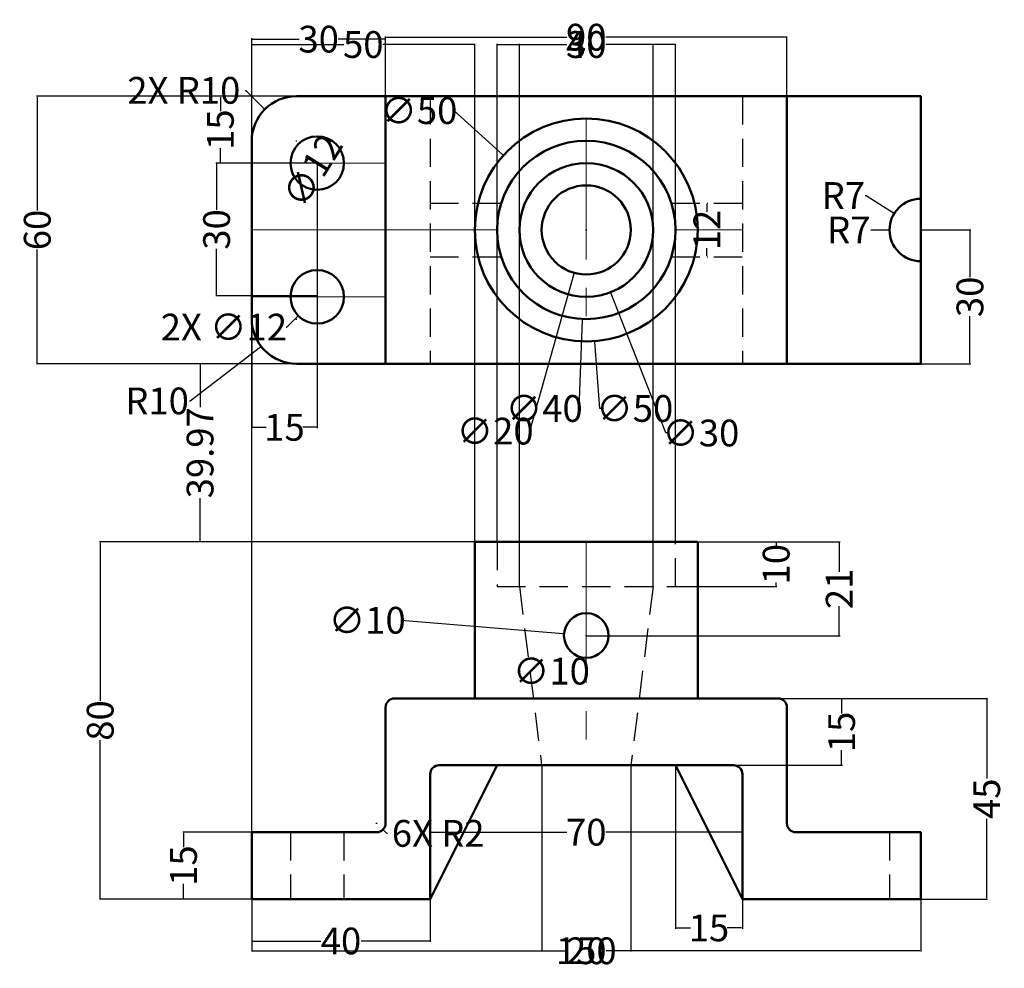
# Model space of a CAD drawing. Units: millimetres. Extents: x 74 to 295, y 59 to 272.
import ezdxf

# ---------------------------------------------------------------- set-up
doc = ezdxf.new("R2010")
doc.units = ezdxf.units.MM
doc.header["$MEASUREMENT"] = 0
doc.linetypes.add('CENTER', pattern=[50.8, 31.75, -6.35, 6.35, -6.35])
doc.linetypes.add('HIDDEN', pattern=[9.525, 6.35, -3.175])
for name, color, linetype, lineweight in [('M-CNTR', 4, 'CENTER', 18), ('M-DIMS', 2, 'Continuous', 25), ('M-HIDN', 3, 'HIDDEN', 25), ('M-OUTL', 7, 'Continuous', 50)]:
    doc.layers.add(name, color=color, linetype=linetype, lineweight=lineweight)
doc.styles.get("Standard").update_dxf_attribs({"font": 'arial.ttf'})
doc.dimstyles.get("Standard").update_dxf_attribs({"dimtxt": 6, "dimasz": 0.18, "dimexe": 0.18, "dimexo": 0.0625, "dimgap": 0.09, "dimtad": 0, "dimtoh": 1, "dimdec": 0, "dimzin": 0, "dimdsep": 46, "dimtxsty": 'Standard', "dimcen": 0.09, "dimadec": 0, "dimazin": 0, "dimtfac": 1, "dimtdec": 0, "dimtofl": 0, "dimtmove": 0, "dimatfit": 3, "dimfxl": 1, "dimtolj": 1, "dimtzin": 0, "dimarcsym": 0})

# ---------------------------------------------------------------- blocks, each defined once
blk = doc.blocks.new('*U1')
at = {"layer": 'M-CNTR', "color": 0, "transparency": 16777216}
blk.add_line((0, 25.12), (0, -25.12), dxfattribs=at)
blk = doc.blocks.new('*D2')
at = {"layer": 'Defpoints', "color": 0, "transparency": 16777216}
for p in [(156.09, 267.91), (126.09, 245.1), (156.09, 245.1)]:
    blk.add_point(p, dxfattribs=at)
at = {"layer": 'M-DIMS', "color": 0, "lineweight": -2, "transparency": 16777216}
for p, q in [((126.09, 245.17), (126.09, 268.09)), ((126.27, 267.91), (136.71, 267.91)), ((155.91, 267.91), (145.46, 267.91)), ((156.09, 245.17), (156.09, 268.09))]:
    blk.add_line(p, q, dxfattribs=at)
at = {"layer": 'M-DIMS', "color": 0, "transparency": 16777216}
for points in [[(126.27, 267.94), (126.27, 267.88), (126.09, 267.91)], [(155.91, 267.94), (155.91, 267.88), (156.09, 267.91)]]:
    blk.add_solid(points, dxfattribs=at)
at = {"layer": 'M-DIMS', "color": 0, "transparency": 16777216, "insert": (141.09, 267.91), "char_height": 6, "attachment_point": 5}
blk.add_mtext('\\A1;30', dxfattribs=at)
blk = doc.blocks.new('*D3')
at = {"layer": 'Defpoints', "color": 0, "transparency": 16777216}
for p in [(246.09, 268.34), (156.09, 255.1), (246.09, 255.1)]:
    blk.add_point(p, dxfattribs=at)
at = {"layer": 'M-DIMS', "color": 0, "lineweight": -2, "transparency": 16777216}
for p, q in [((156.09, 255.17), (156.09, 268.52)), ((156.27, 268.34), (196.71, 268.34)), ((245.91, 268.34), (205.46, 268.34)), ((246.09, 255.17), (246.09, 268.52))]:
    blk.add_line(p, q, dxfattribs=at)
at = {"layer": 'M-DIMS', "color": 0, "transparency": 16777216}
for points in [[(156.27, 268.37), (156.27, 268.31), (156.09, 268.34)], [(245.91, 268.37), (245.91, 268.31), (246.09, 268.34)]]:
    blk.add_solid(points, dxfattribs=at)
at = {"layer": 'M-DIMS', "color": 0, "transparency": 16777216, "insert": (201.09, 268.34), "char_height": 6, "attachment_point": 5}
blk.add_mtext('\\A1;90', dxfattribs=at)
blk = doc.blocks.new('*D4')
at = {"layer": 'Defpoints', "color": 0, "transparency": 16777216}
for p in [(228.13, 231.1), (228.13, 231.1), (228.13, 219.1)]:
    blk.add_point(p, dxfattribs=at)
at = {"layer": 'M-DIMS', "color": 0, "lineweight": -2, "transparency": 16777216}
for p, q in [((228.13, 230.92), (228.13, 229.18)), ((228.19, 231.1), (228.31, 231.1)), ((228.13, 219.28), (228.13, 221.03)), ((228.19, 219.1), (228.31, 219.1))]:
    blk.add_line(p, q, dxfattribs=at)
at = {"layer": 'M-DIMS', "color": 0, "transparency": 16777216}
for points in [[(228.1, 230.92), (228.16, 230.92), (228.13, 231.1)], [(228.1, 219.28), (228.16, 219.28), (228.13, 219.1)]]:
    blk.add_solid(points, dxfattribs=at)
at = {"layer": 'M-DIMS', "color": 0, "transparency": 16777216, "insert": (228.13, 225.1), "char_height": 6, "attachment_point": 5, "rotation": 90}
blk.add_mtext('\\A1;12', dxfattribs=at)
blk = doc.blocks.new('*D5')
at = {"layer": 'Defpoints', "color": 0, "transparency": 16777216}
for p in [(276.09, 225.1), (276.09, 195.1), (287.11, 195.1)]:
    blk.add_point(p, dxfattribs=at)
at = {"layer": 'M-DIMS', "color": 0, "lineweight": -2, "transparency": 16777216}
for p, q in [((276.15, 225.1), (287.29, 225.1)), ((287.11, 224.92), (287.11, 214.48)), ((287.11, 195.28), (287.11, 205.73)), ((276.15, 195.1), (287.29, 195.1))]:
    blk.add_line(p, q, dxfattribs=at)
at = {"layer": 'M-DIMS', "color": 0, "transparency": 16777216}
for points in [[(287.08, 224.92), (287.14, 224.92), (287.11, 225.1)], [(287.08, 195.28), (287.14, 195.28), (287.11, 195.1)]]:
    blk.add_solid(points, dxfattribs=at)
at = {"layer": 'M-DIMS', "color": 0, "transparency": 16777216, "insert": (287.11, 210.1), "char_height": 6, "attachment_point": 5, "rotation": 90}
blk.add_mtext('\\A1;30', dxfattribs=at)
blk = doc.blocks.new('*D6')
at = {"layer": 'Defpoints', "color": 0, "transparency": 16777216}
for p in [(126.09, 240.1), (140.77, 240.1), (126.09, 180.83)]:
    blk.add_point(p, dxfattribs=at)
at = {"layer": 'M-DIMS', "color": 0, "lineweight": -2, "transparency": 16777216}
for p, q in [((126.09, 240.04), (126.09, 180.65)), ((140.77, 240.04), (140.77, 180.65)), ((126.27, 180.83), (129.3, 180.83)), ((140.59, 180.83), (137.55, 180.83))]:
    blk.add_line(p, q, dxfattribs=at)
at = {"layer": 'M-DIMS', "color": 0, "transparency": 16777216}
for points in [[(126.27, 180.86), (126.27, 180.8), (126.09, 180.83)], [(140.59, 180.86), (140.59, 180.8), (140.77, 180.83)]]:
    blk.add_solid(points, dxfattribs=at)
at = {"layer": 'M-DIMS', "color": 0, "transparency": 16777216, "insert": (133.43, 180.83), "char_height": 6, "attachment_point": 5}
blk.add_mtext('\\A1;15', dxfattribs=at)
blk = doc.blocks.new('*D7')
at = {"layer": 'Defpoints', "color": 0, "transparency": 16777216}
for p in [(119.05, 255.1), (141.09, 255.1), (141.09, 240.1)]:
    blk.add_point(p, dxfattribs=at)
at = {"layer": 'M-DIMS', "color": 0, "lineweight": -2, "transparency": 16777216}
for p, q in [((141.02, 255.1), (118.87, 255.1)), ((119.05, 254.92), (119.05, 251.73)), ((119.05, 240.28), (119.05, 243.48)), ((141.02, 240.1), (118.87, 240.1))]:
    blk.add_line(p, q, dxfattribs=at)
at = {"layer": 'M-DIMS', "color": 0, "transparency": 16777216}
for points in [[(119.02, 254.92), (119.08, 254.92), (119.05, 255.1)], [(119.02, 240.28), (119.08, 240.28), (119.05, 240.1)]]:
    blk.add_solid(points, dxfattribs=at)
at = {"layer": 'M-DIMS', "color": 0, "transparency": 16777216, "insert": (119.05, 247.6), "char_height": 6, "attachment_point": 5, "rotation": 90}
blk.add_mtext('\\A1;15', dxfattribs=at)
blk = doc.blocks.new('*D8')
at = {"layer": 'Defpoints', "color": 0, "transparency": 16777216}
for p in [(140.77, 240.1), (118.2, 210.34), (140.77, 210.34)]:
    blk.add_point(p, dxfattribs=at)
at = {"layer": 'M-DIMS', "color": 0, "lineweight": -2, "transparency": 16777216}
for p, q in [((140.7, 240.1), (118.02, 240.1)), ((118.2, 239.92), (118.2, 229.6)), ((118.2, 210.52), (118.2, 220.85)), ((140.7, 210.34), (118.02, 210.34))]:
    blk.add_line(p, q, dxfattribs=at)
at = {"layer": 'M-DIMS', "color": 0, "transparency": 16777216}
for points in [[(118.17, 239.92), (118.23, 239.92), (118.2, 240.1)], [(118.17, 210.52), (118.23, 210.52), (118.2, 210.34)]]:
    blk.add_solid(points, dxfattribs=at)
at = {"layer": 'M-DIMS', "color": 0, "transparency": 16777216, "insert": (118.2, 225.22), "char_height": 6, "attachment_point": 5, "rotation": 90}
blk.add_mtext('\\A1;30', dxfattribs=at)
blk = doc.blocks.new('*D9')
at = {"layer": 'Defpoints', "color": 0, "transparency": 16777216}
for p in [(270.16, 228.83), (276.09, 225.1)]:
    blk.add_point(p, dxfattribs=at)
at = {"layer": 'M-DIMS', "color": 0, "lineweight": -2, "transparency": 16777216}
for p, q in [((263.64, 232.83), (263.82, 232.83)), ((263.82, 232.83), (270.01, 228.93)), ((276.09, 225.01), (276.09, 225.19)), ((276, 225.1), (276.18, 225.1))]:
    blk.add_line(p, q, dxfattribs=at)
at = {"layer": 'M-DIMS', "color": 0, "transparency": 16777216}
blk.add_solid([(270.03, 228.95), (270, 228.9), (270.16, 228.83)], dxfattribs=at)
at = {"layer": 'M-DIMS', "color": 0, "transparency": 16777216, "insert": (258.72, 232.83), "char_height": 6, "attachment_point": 5}
blk.add_mtext('\\A1;R7', dxfattribs=at)
blk = doc.blocks.new('*D10')
at = {"layer": 'Defpoints', "color": 0, "transparency": 16777216}
for p in [(143.95, 245.19), (137.58, 235.02)]:
    blk.add_point(p, dxfattribs=at)
at = {"layer": 'M-DIMS', "color": 0, "lineweight": -2, "transparency": 16777216}
blk.add_line((143.76, 244.88), (143.85, 245.04), dxfattribs=at)
at = {"layer": 'M-DIMS', "color": 0, "transparency": 16777216}
blk.add_solid([(143.83, 245.05), (143.88, 245.02), (143.95, 245.19)], dxfattribs=at)
at = {"layer": 'M-DIMS', "color": 0, "transparency": 16777216, "insert": (139.72, 238.42), "char_height": 6, "attachment_point": 5, "rotation": 57.9702}
blk.add_mtext('\\A1;∅12', dxfattribs=at)
blk = doc.blocks.new('*D11')
at = {"layer": 'Defpoints', "color": 0, "transparency": 16777216}
for p in [(136.09, 255.1), (77.99, 195.1), (136.09, 195.1)]:
    blk.add_point(p, dxfattribs=at)
at = {"layer": 'M-DIMS', "color": 0, "lineweight": -2, "transparency": 16777216}
for p, q in [((136.02, 255.1), (77.81, 255.1)), ((77.99, 254.92), (77.99, 229.5)), ((77.99, 195.28), (77.99, 220.71)), ((136.02, 195.1), (77.81, 195.1))]:
    blk.add_line(p, q, dxfattribs=at)
at = {"layer": 'M-DIMS', "color": 0, "transparency": 16777216}
for points in [[(77.96, 254.92), (78.02, 254.92), (77.99, 255.1)], [(77.96, 195.28), (78.02, 195.28), (77.99, 195.1)]]:
    blk.add_solid(points, dxfattribs=at)
at = {"layer": 'M-DIMS', "color": 0, "transparency": 16777216, "insert": (77.99, 225.1), "char_height": 6, "attachment_point": 5, "rotation": 90}
blk.add_mtext('\\A1;60', dxfattribs=at)
blk = doc.blocks.new('*D12')
at = {"layer": 'Defpoints', "color": 0, "transparency": 16777216}
for p in [(203.78, 234.73), (198.4, 215.47)]:
    blk.add_point(p, dxfattribs=at)
at = {"layer": 'M-DIMS', "color": 0, "lineweight": -2, "transparency": 16777216}
for p, q in [((201.09, 225.01), (201.09, 225.19)), ((201, 225.1), (201.18, 225.1)), ((188.47, 179.98), (198.35, 215.3)), ((188.29, 179.98), (188.47, 179.98))]:
    blk.add_line(p, q, dxfattribs=at)
at = {"layer": 'M-DIMS', "color": 0, "transparency": 16777216}
blk.add_solid([(198.32, 215.31), (198.38, 215.29), (198.4, 215.47)], dxfattribs=at)
at = {"layer": 'M-DIMS', "color": 0, "transparency": 16777216, "insert": (180.65, 179.98), "char_height": 6, "attachment_point": 5}
blk.add_mtext('\\A1;∅20', dxfattribs=at)
blk = doc.blocks.new('*D13')
at = {"layer": 'Defpoints', "color": 0, "transparency": 16777216}
for p in [(195.61, 239.07), (206.57, 211.14)]:
    blk.add_point(p, dxfattribs=at)
at = {"layer": 'M-DIMS', "color": 0, "lineweight": -2, "transparency": 16777216}
for p, q in [((201.09, 225.01), (201.09, 225.19)), ((201, 225.1), (201.18, 225.1)), ((218.95, 179.56), (206.63, 210.97)), ((219.13, 179.56), (218.95, 179.56))]:
    blk.add_line(p, q, dxfattribs=at)
at = {"layer": 'M-DIMS', "color": 0, "transparency": 16777216}
blk.add_solid([(206.66, 210.98), (206.6, 210.96), (206.57, 211.14)], dxfattribs=at)
at = {"layer": 'M-DIMS', "color": 0, "transparency": 16777216, "insert": (226.77, 179.56), "char_height": 6, "attachment_point": 5}
blk.add_mtext('\\A1;∅30', dxfattribs=at)
blk = doc.blocks.new('*D14')
at = {"layer": 'Defpoints', "color": 0, "transparency": 16777216}
for p in [(201.89, 245.09), (200.29, 205.12)]:
    blk.add_point(p, dxfattribs=at)
at = {"layer": 'M-DIMS', "color": 0, "lineweight": -2, "transparency": 16777216}
for p, q in [((201.09, 225.01), (201.09, 225.19)), ((201, 225.1), (201.18, 225.1)), ((199.48, 185.06), (200.28, 204.94)), ((199.3, 185.06), (199.48, 185.06))]:
    blk.add_line(p, q, dxfattribs=at)
at = {"layer": 'M-DIMS', "color": 0, "transparency": 16777216}
blk.add_solid([(200.25, 204.94), (200.31, 204.94), (200.29, 205.12)], dxfattribs=at)
at = {"layer": 'M-DIMS', "color": 0, "transparency": 16777216, "insert": (191.66, 185.06), "char_height": 6, "attachment_point": 5}
blk.add_mtext('\\A1;∅40', dxfattribs=at)
blk = doc.blocks.new('*D15')
at = {"layer": 'Defpoints', "color": 0, "transparency": 16777216}
for p in [(199.19, 250.03), (202.99, 200.17)]:
    blk.add_point(p, dxfattribs=at)
at = {"layer": 'M-DIMS', "color": 0, "lineweight": -2, "transparency": 16777216}
for p, q in [((201.09, 225.01), (201.09, 225.19)), ((201, 225.1), (201.18, 225.1)), ((204.14, 185.06), (203, 200)), ((204.32, 185.06), (204.14, 185.06))]:
    blk.add_line(p, q, dxfattribs=at)
at = {"layer": 'M-DIMS', "color": 0, "transparency": 16777216}
blk.add_solid([(203.03, 200), (202.97, 199.99), (202.99, 200.17)], dxfattribs=at)
at = {"layer": 'M-DIMS', "color": 0, "transparency": 16777216, "insert": (211.96, 185.06), "char_height": 6, "attachment_point": 5}
blk.add_mtext('\\A1;∅50', dxfattribs=at)
blk = doc.blocks.new('*D16')
at = {"layer": 'Defpoints', "color": 0, "transparency": 16777216}
for p in [(136.09, 205.1), (128.17, 199)]:
    blk.add_point(p, dxfattribs=at)
at = {"layer": 'M-DIMS', "color": 0, "lineweight": -2, "transparency": 16777216}
for p, q in [((136, 205.1), (136.18, 205.1)), ((136.09, 205.01), (136.09, 205.19)), ((112.28, 186.75), (128.02, 198.89)), ((112.1, 186.75), (112.28, 186.75))]:
    blk.add_line(p, q, dxfattribs=at)
at = {"layer": 'M-DIMS', "color": 0, "transparency": 16777216}
blk.add_solid([(128.01, 198.91), (128.04, 198.86), (128.17, 199)], dxfattribs=at)
at = {"layer": 'M-DIMS', "color": 0, "transparency": 16777216, "insert": (104.85, 186.75), "char_height": 6, "attachment_point": 5}
blk.add_mtext('\\A1;R10', dxfattribs=at)
blk = doc.blocks.new('*D17')
at = {"layer": 'Defpoints', "color": 0, "transparency": 16777216}
for p in [(196.1, 134.54), (206.07, 133.72)]:
    blk.add_point(p, dxfattribs=at)
at = {"layer": 'M-DIMS', "color": 0, "lineweight": -2, "transparency": 16777216}
for p, q in [((159.61, 137.55), (195.92, 134.56)), ((201, 134.13), (201.18, 134.13)), ((201.09, 134.04), (201.09, 134.22))]:
    blk.add_line(p, q, dxfattribs=at)
at = {"layer": 'M-DIMS', "color": 0, "transparency": 16777216}
blk.add_solid([(195.93, 134.59), (195.92, 134.53), (196.1, 134.54)], dxfattribs=at)
at = {"layer": 'M-DIMS', "color": 0, "transparency": 16777216, "insert": (151.97, 137.55), "char_height": 6, "attachment_point": 5}
blk.add_mtext('\\A1;∅10', dxfattribs=at)
blk = doc.blocks.new('*D18')
at = {"layer": 'Defpoints', "color": 0, "transparency": 16777216}
for p in [(221.09, 155.13), (243.66, 155.13), (221.09, 145.13)]:
    blk.add_point(p, dxfattribs=at)
at = {"layer": 'M-DIMS', "color": 0, "lineweight": -2, "transparency": 16777216}
for p, q in [((221.15, 155.13), (243.84, 155.13)), ((243.66, 154.95), (243.66, 154.23)), ((243.66, 145.31), (243.66, 146.04)), ((221.15, 145.13), (243.84, 145.13))]:
    blk.add_line(p, q, dxfattribs=at)
at = {"layer": 'M-DIMS', "color": 0, "transparency": 16777216}
for points in [[(243.63, 154.95), (243.69, 154.95), (243.66, 155.13)], [(243.63, 145.31), (243.69, 145.31), (243.66, 145.13)]]:
    blk.add_solid(points, dxfattribs=at)
at = {"layer": 'M-DIMS', "color": 0, "transparency": 16777216, "insert": (243.66, 150.13), "char_height": 6, "attachment_point": 5, "rotation": 90}
blk.add_mtext('\\A1;10', dxfattribs=at)
blk = doc.blocks.new('*D19')
at = {"layer": 'Defpoints', "color": 0, "transparency": 16777216}
for p in [(201.09, 155.13), (257.8, 155.13), (201.09, 134.04)]:
    blk.add_point(p, dxfattribs=at)
at = {"layer": 'M-DIMS', "color": 0, "lineweight": -2, "transparency": 16777216}
for p, q in [((201.15, 155.13), (257.98, 155.13)), ((257.8, 154.95), (257.8, 148.45)), ((257.8, 134.22), (257.8, 140.73)), ((201.15, 134.04), (257.98, 134.04))]:
    blk.add_line(p, q, dxfattribs=at)
at = {"layer": 'M-DIMS', "color": 0, "transparency": 16777216}
for points in [[(257.77, 154.95), (257.83, 154.95), (257.8, 155.13)], [(257.77, 134.22), (257.83, 134.22), (257.8, 134.04)]]:
    blk.add_solid(points, dxfattribs=at)
at = {"layer": 'M-DIMS', "color": 0, "transparency": 16777216, "insert": (257.8, 144.59), "char_height": 6, "attachment_point": 5, "rotation": 90}
blk.add_mtext('\\A1;21', dxfattribs=at)
blk = doc.blocks.new('*D20')
at = {"layer": 'Defpoints', "color": 0, "transparency": 16777216}
for p in [(234.09, 120.01), (258.33, 120.01), (234.09, 105.01)]:
    blk.add_point(p, dxfattribs=at)
at = {"layer": 'M-DIMS', "color": 0, "lineweight": -2, "transparency": 16777216}
for p, q in [((234.15, 120.01), (258.51, 120.01)), ((258.33, 119.83), (258.33, 116.64)), ((258.33, 105.19), (258.33, 108.39)), ((234.15, 105.01), (258.51, 105.01))]:
    blk.add_line(p, q, dxfattribs=at)
at = {"layer": 'M-DIMS', "color": 0, "transparency": 16777216}
for points in [[(258.3, 119.83), (258.36, 119.83), (258.33, 120.01)], [(258.3, 105.19), (258.36, 105.19), (258.33, 105.01)]]:
    blk.add_solid(points, dxfattribs=at)
at = {"layer": 'M-DIMS', "color": 0, "transparency": 16777216, "insert": (258.33, 112.51), "char_height": 6, "attachment_point": 5, "rotation": 90}
blk.add_mtext('\\A1;15', dxfattribs=at)
blk = doc.blocks.new('*D21')
at = {"layer": 'Defpoints', "color": 0, "transparency": 16777216}
for p in [(126.09, 75.01), (166.09, 75.01), (166.09, 65.6)]:
    blk.add_point(p, dxfattribs=at)
at = {"layer": 'M-DIMS', "color": 0, "lineweight": -2, "transparency": 16777216}
for p, q in [((126.09, 74.95), (126.09, 65.42)), ((166.09, 74.95), (166.09, 65.42)), ((126.27, 65.6), (141.59, 65.6)), ((165.91, 65.6), (150.59, 65.6))]:
    blk.add_line(p, q, dxfattribs=at)
at = {"layer": 'M-DIMS', "color": 0, "transparency": 16777216}
for points in [[(126.27, 65.63), (126.27, 65.57), (126.09, 65.6)], [(165.91, 65.63), (165.91, 65.57), (166.09, 65.6)]]:
    blk.add_solid(points, dxfattribs=at)
at = {"layer": 'M-DIMS', "color": 0, "transparency": 16777216, "insert": (146.09, 65.6), "char_height": 6, "attachment_point": 5}
blk.add_mtext('\\A1;40', dxfattribs=at)
blk = doc.blocks.new('*D22')
at = {"layer": 'Defpoints', "color": 0, "transparency": 16777216}
for p in [(221.09, 105.01), (236.09, 89.01), (236.09, 68.54)]:
    blk.add_point(p, dxfattribs=at)
at = {"layer": 'M-DIMS', "color": 0, "lineweight": -2, "transparency": 16777216}
for p, q in [((221.09, 104.95), (221.09, 68.36)), ((236.09, 88.95), (236.09, 68.36)), ((221.27, 68.54), (224.46, 68.54)), ((235.91, 68.54), (232.71, 68.54))]:
    blk.add_line(p, q, dxfattribs=at)
at = {"layer": 'M-DIMS', "color": 0, "transparency": 16777216}
for points in [[(221.27, 68.57), (221.27, 68.51), (221.09, 68.54)], [(235.91, 68.57), (235.91, 68.51), (236.09, 68.54)]]:
    blk.add_solid(points, dxfattribs=at)
at = {"layer": 'M-DIMS', "color": 0, "transparency": 16777216, "insert": (228.59, 68.54), "char_height": 6, "attachment_point": 5}
blk.add_mtext('\\A1;15', dxfattribs=at)
blk = doc.blocks.new('*D23')
at = {"layer": 'Defpoints', "color": 0, "transparency": 16777216}
for p in [(244.09, 120.01), (244.09, 75.01), (290.88, 75.01)]:
    blk.add_point(p, dxfattribs=at)
at = {"layer": 'M-DIMS', "color": 0, "lineweight": -2, "transparency": 16777216}
for p, q in [((244.15, 120.01), (291.06, 120.01)), ((290.88, 119.83), (290.88, 102.04)), ((290.88, 75.19), (290.88, 92.98)), ((244.15, 75.01), (291.06, 75.01))]:
    blk.add_line(p, q, dxfattribs=at)
at = {"layer": 'M-DIMS', "color": 0, "transparency": 16777216}
for points in [[(290.85, 119.83), (290.91, 119.83), (290.88, 120.01)], [(290.85, 75.19), (290.91, 75.19), (290.88, 75.01)]]:
    blk.add_solid(points, dxfattribs=at)
at = {"layer": 'M-DIMS', "color": 0, "transparency": 16777216, "insert": (290.88, 97.51), "char_height": 6, "attachment_point": 5, "rotation": 90}
blk.add_mtext('\\A1;45', dxfattribs=at)
blk = doc.blocks.new('*D24')
at = {"layer": 'Defpoints', "color": 0, "transparency": 16777216}
for p in [(126.09, 90.01), (110.78, 75.01), (126.09, 75.01)]:
    blk.add_point(p, dxfattribs=at)
at = {"layer": 'M-DIMS', "color": 0, "lineweight": -2, "transparency": 16777216}
for p, q in [((126.02, 90.01), (110.6, 90.01)), ((110.78, 89.83), (110.78, 86.64)), ((110.78, 75.19), (110.78, 78.39)), ((126.02, 75.01), (110.6, 75.01))]:
    blk.add_line(p, q, dxfattribs=at)
at = {"layer": 'M-DIMS', "color": 0, "transparency": 16777216}
for points in [[(110.75, 89.83), (110.81, 89.83), (110.78, 90.01)], [(110.75, 75.19), (110.81, 75.19), (110.78, 75.01)]]:
    blk.add_solid(points, dxfattribs=at)
at = {"layer": 'M-DIMS', "color": 0, "transparency": 16777216, "insert": (110.78, 82.51), "char_height": 6, "attachment_point": 5, "rotation": 90}
blk.add_mtext('\\A1;15', dxfattribs=at)
blk = doc.blocks.new('*D25')
at = {"layer": 'Defpoints', "color": 0, "transparency": 16777216}
for p in [(236.09, 90.01), (166.09, 75.01), (236.09, 75.01)]:
    blk.add_point(p, dxfattribs=at)
at = {"layer": 'M-DIMS', "color": 0, "lineweight": -2, "transparency": 16777216}
for p, q in [((166.09, 75.08), (166.09, 90.19)), ((166.27, 90.01), (196.73, 90.01)), ((235.91, 90.01), (205.44, 90.01)), ((236.09, 75.08), (236.09, 90.19))]:
    blk.add_line(p, q, dxfattribs=at)
at = {"layer": 'M-DIMS', "color": 0, "transparency": 16777216}
for points in [[(166.27, 90.04), (166.27, 89.98), (166.09, 90.01)], [(235.91, 90.04), (235.91, 89.98), (236.09, 90.01)]]:
    blk.add_solid(points, dxfattribs=at)
at = {"layer": 'M-DIMS', "color": 0, "transparency": 16777216, "insert": (201.09, 90.01), "char_height": 6, "attachment_point": 5}
blk.add_mtext('\\A1;70', dxfattribs=at)
blk = doc.blocks.new('*D26')
at = {"layer": 'Defpoints', "color": 0, "transparency": 16777216}
for p in [(176.09, 155.13), (92.1, 75.01), (166.09, 75.01)]:
    blk.add_point(p, dxfattribs=at)
at = {"layer": 'M-DIMS', "color": 0, "lineweight": -2, "transparency": 16777216}
for p, q in [((176.02, 155.13), (91.92, 155.13)), ((92.1, 154.95), (92.1, 119.45)), ((92.1, 75.19), (92.1, 110.69)), ((166.02, 75.01), (91.92, 75.01))]:
    blk.add_line(p, q, dxfattribs=at)
at = {"layer": 'M-DIMS', "color": 0, "transparency": 16777216}
for points in [[(92.07, 154.95), (92.13, 154.95), (92.1, 155.13)], [(92.07, 75.19), (92.13, 75.19), (92.1, 75.01)]]:
    blk.add_solid(points, dxfattribs=at)
at = {"layer": 'M-DIMS', "color": 0, "transparency": 16777216, "insert": (92.1, 115.07), "char_height": 6, "attachment_point": 5, "rotation": 90}
blk.add_mtext('\\A1;80', dxfattribs=at)
blk = doc.blocks.new('MOUNT-HOLE-D12')
blk.add_circle((0, 0), 6)
blk = doc.blocks.new('*D28')
at = {"layer": 'Defpoints', "color": 0, "transparency": 16777216}
for p in [(126.09, 75.01), (276.09, 75.01), (276.09, 63.41)]:
    blk.add_point(p, dxfattribs=at)
at = {"layer": 'M-DIMS', "color": 0, "lineweight": -2, "transparency": 16777216}
for p, q in [((126.09, 74.95), (126.09, 63.23)), ((276.09, 74.95), (276.09, 63.23)), ((126.27, 63.41), (194.66, 63.41)), ((275.91, 63.41), (207.51, 63.41))]:
    blk.add_line(p, q, dxfattribs=at)
at = {"layer": 'M-DIMS', "color": 0, "transparency": 16777216}
for points in [[(126.27, 63.44), (126.27, 63.38), (126.09, 63.41)], [(275.91, 63.44), (275.91, 63.38), (276.09, 63.41)]]:
    blk.add_solid(points, dxfattribs=at)
at = {"layer": 'M-DIMS', "color": 0, "transparency": 16777216, "insert": (201.09, 63.41), "char_height": 6, "attachment_point": 5}
blk.add_mtext('\\A1;150', dxfattribs=at)
blk = doc.blocks.new('*D29')
at = {"layer": 'Defpoints', "color": 0, "transparency": 16777216}
for p in [(126.09, 266.7), (176.09, 155.13), (126.09, 90.01)]:
    blk.add_point(p, dxfattribs=at)
at = {"layer": 'M-DIMS', "color": 0, "lineweight": -2, "transparency": 16777216}
for p, q in [((126.09, 90.08), (126.09, 266.88)), ((126.27, 266.7), (146.71, 266.7)), ((175.91, 266.7), (155.46, 266.7)), ((176.09, 155.2), (176.09, 266.88))]:
    blk.add_line(p, q, dxfattribs=at)
at = {"layer": 'M-DIMS', "color": 0, "transparency": 16777216}
for points in [[(126.27, 266.73), (126.27, 266.67), (126.09, 266.7)], [(175.91, 266.73), (175.91, 266.67), (176.09, 266.7)]]:
    blk.add_solid(points, dxfattribs=at)
at = {"layer": 'M-DIMS', "color": 0, "transparency": 16777216, "insert": (151.09, 266.7), "char_height": 6, "attachment_point": 5}
blk.add_mtext('\\A1;50', dxfattribs=at)
blk = doc.blocks.new('*D30')
at = {"layer": 'Defpoints', "color": 0, "transparency": 16777216}
for p in [(221.09, 266.7), (181.09, 155.13), (221.09, 155.13)]:
    blk.add_point(p, dxfattribs=at)
at = {"layer": 'M-DIMS', "color": 0, "lineweight": -2, "transparency": 16777216}
for p, q in [((181.09, 155.2), (181.09, 266.88)), ((181.27, 266.7), (196.59, 266.7)), ((220.91, 266.7), (205.59, 266.7)), ((221.09, 155.2), (221.09, 266.88))]:
    blk.add_line(p, q, dxfattribs=at)
at = {"layer": 'M-DIMS', "color": 0, "transparency": 16777216}
for points in [[(181.27, 266.73), (181.27, 266.67), (181.09, 266.7)], [(220.91, 266.73), (220.91, 266.67), (221.09, 266.7)]]:
    blk.add_solid(points, dxfattribs=at)
at = {"layer": 'M-DIMS', "color": 0, "transparency": 16777216, "insert": (201.09, 266.7), "char_height": 6, "attachment_point": 5}
blk.add_mtext('\\A1;40', dxfattribs=at)
blk = doc.blocks.new('*D31')
at = {"layer": 'Defpoints', "color": 0, "transparency": 16777216}
for p in [(216.09, 266.7), (186.09, 145.13), (216.09, 145.13)]:
    blk.add_point(p, dxfattribs=at)
at = {"layer": 'M-DIMS', "color": 0, "lineweight": -2, "transparency": 16777216}
for p, q in [((186.09, 145.2), (186.09, 266.88)), ((186.27, 266.7), (196.71, 266.7)), ((215.91, 266.7), (205.46, 266.7)), ((216.09, 145.2), (216.09, 266.88))]:
    blk.add_line(p, q, dxfattribs=at)
at = {"layer": 'M-DIMS', "color": 0, "transparency": 16777216}
for points in [[(186.27, 266.73), (186.27, 266.67), (186.09, 266.7)], [(215.91, 266.73), (215.91, 266.67), (216.09, 266.7)]]:
    blk.add_solid(points, dxfattribs=at)
at = {"layer": 'M-DIMS', "color": 0, "transparency": 16777216, "insert": (201.09, 266.7), "char_height": 6, "attachment_point": 5}
blk.add_mtext('\\A1;30', dxfattribs=at)
blk = doc.blocks.new('*D32')
at = {"layer": 'Defpoints', "color": 0, "transparency": 16777216}
for p in [(191.09, 105.01), (211.09, 105.01), (211.09, 63.41)]:
    blk.add_point(p, dxfattribs=at)
at = {"layer": 'M-DIMS', "color": 0, "lineweight": -2, "transparency": 16777216}
for p, q in [((191.09, 104.95), (191.09, 63.23)), ((211.09, 104.95), (211.09, 63.23)), ((191.27, 63.41), (196.66, 63.41)), ((210.91, 63.41), (205.52, 63.41))]:
    blk.add_line(p, q, dxfattribs=at)
at = {"layer": 'M-DIMS', "color": 0, "transparency": 16777216}
for points in [[(191.27, 63.44), (191.27, 63.38), (191.09, 63.41)], [(210.91, 63.44), (210.91, 63.38), (211.09, 63.41)]]:
    blk.add_solid(points, dxfattribs=at)
at = {"layer": 'M-DIMS', "color": 0, "transparency": 16777216, "insert": (201.09, 63.41), "char_height": 6, "attachment_point": 5}
blk.add_mtext('\\A1;20', dxfattribs=at)
blk = doc.blocks.new('*D33')
at = {"layer": 'Defpoints', "color": 0, "transparency": 16777216}
for p in [(156.09, 195.1), (114.49, 155.13), (176.09, 155.13)]:
    blk.add_point(p, dxfattribs=at)
at = {"layer": 'M-DIMS', "color": 0, "lineweight": -2, "transparency": 16777216}
for p, q in [((156.02, 195.1), (114.31, 195.1)), ((114.49, 194.92), (114.49, 185.33)), ((114.49, 155.31), (114.49, 164.91)), ((176.02, 155.13), (114.31, 155.13))]:
    blk.add_line(p, q, dxfattribs=at)
at = {"layer": 'M-DIMS', "color": 0, "transparency": 16777216}
for points in [[(114.46, 194.92), (114.52, 194.92), (114.49, 195.1)], [(114.46, 155.31), (114.52, 155.31), (114.49, 155.13)]]:
    blk.add_solid(points, dxfattribs=at)
at = {"layer": 'M-DIMS', "color": 0, "transparency": 16777216, "insert": (114.49, 175.12), "char_height": 6, "attachment_point": 5, "rotation": 90}
blk.add_mtext('\\A1;39.97', dxfattribs=at)
blk = doc.blocks.new('*D34')
at = {"layer": 'Defpoints', "color": 0, "transparency": 16777216}
for p in [(182.52, 241.84), (219.66, 208.36)]:
    blk.add_point(p, dxfattribs=at)
at = {"layer": 'M-DIMS', "color": 0, "lineweight": -2, "transparency": 16777216}
for p, q in [((171.2, 251.88), (171.38, 251.88)), ((171.38, 251.88), (182.38, 241.96)), ((201.09, 225.01), (201.09, 225.19)), ((201, 225.1), (201.18, 225.1))]:
    blk.add_line(p, q, dxfattribs=at)
at = {"layer": 'M-DIMS', "color": 0, "transparency": 16777216}
blk.add_solid([(182.4, 241.98), (182.36, 241.94), (182.52, 241.84)], dxfattribs=at)
at = {"layer": 'M-DIMS', "color": 0, "transparency": 16777216, "insert": (163.56, 251.88), "char_height": 6, "attachment_point": 5}
blk.add_mtext('\\A1;∅50', dxfattribs=at)
blk = doc.blocks.new('*D35')
at = {"layer": 'Defpoints', "color": 0, "transparency": 16777216}
for p in [(129.02, 252.17), (136.09, 245.1)]:
    blk.add_point(p, dxfattribs=at)
at = {"layer": 'M-DIMS', "color": 0, "lineweight": -2, "transparency": 16777216}
for p, q in [((124.59, 256.42), (124.77, 256.42)), ((124.77, 256.42), (128.89, 252.3)), ((136, 245.1), (136.18, 245.1)), ((136.09, 245.01), (136.09, 245.19))]:
    blk.add_line(p, q, dxfattribs=at)
at = {"layer": 'M-DIMS', "color": 0, "transparency": 16777216}
blk.add_solid([(128.91, 252.32), (128.87, 252.28), (129.02, 252.17)], dxfattribs=at)
at = {"layer": 'M-DIMS', "color": 0, "transparency": 16777216, "insert": (110.85, 256.42), "char_height": 6, "attachment_point": 5}
blk.add_mtext('\\A1;2X R10', dxfattribs=at)
blk = doc.blocks.new('*D36')
at = {"layer": 'Defpoints', "color": 0, "transparency": 16777216}
for p in [(269.09, 225.1), (276.09, 225.1)]:
    blk.add_point(p, dxfattribs=at)
at = {"layer": 'M-DIMS', "color": 0, "lineweight": -2, "transparency": 16777216}
for p, q in [((276.09, 225.01), (276.09, 225.19)), ((264.89, 225.1), (268.91, 225.1)), ((276, 225.1), (276.18, 225.1))]:
    blk.add_line(p, q, dxfattribs=at)
at = {"layer": 'M-DIMS', "color": 0, "transparency": 16777216}
blk.add_solid([(268.91, 225.13), (268.91, 225.07), (269.09, 225.1)], dxfattribs=at)
at = {"layer": 'M-DIMS', "color": 0, "transparency": 16777216, "insert": (259.96, 225.1), "char_height": 6, "attachment_point": 5}
blk.add_mtext('\\A1;R7', dxfattribs=at)
blk = doc.blocks.new('*D37')
at = {"layer": 'Defpoints', "color": 0, "transparency": 16777216}
for p in [(145.01, 214.35), (136.52, 205.86)]:
    blk.add_point(p, dxfattribs=at)
at = {"layer": 'M-DIMS', "color": 0, "lineweight": -2, "transparency": 16777216}
for p, q in [((140.68, 210.1), (140.86, 210.1)), ((140.77, 210.01), (140.77, 210.19)), ((133.98, 203.31), (136.4, 205.73)), ((133.8, 203.31), (133.98, 203.31))]:
    blk.add_line(p, q, dxfattribs=at)
at = {"layer": 'M-DIMS', "color": 0, "transparency": 16777216}
blk.add_solid([(136.38, 205.75), (136.42, 205.71), (136.52, 205.86)], dxfattribs=at)
at = {"layer": 'M-DIMS', "color": 0, "transparency": 16777216, "insert": (119.84, 203.31), "char_height": 6, "attachment_point": 5}
blk.add_mtext('\\A1;2X ∅12', dxfattribs=at)
blk = doc.blocks.new('*D38')
at = {"layer": 'Defpoints', "color": 0, "transparency": 16777216}
for p in [(201.09, 139.13), (201.09, 129.13)]:
    blk.add_point(p, dxfattribs=at)
at = {"layer": 'M-DIMS', "color": 0, "lineweight": -2, "transparency": 16777216}
for p, q in [((201, 134.13), (201.18, 134.13)), ((201.09, 134.04), (201.09, 134.22)), ((201.09, 126.13), (201.09, 128.95)), ((200.91, 126.13), (201.09, 126.13))]:
    blk.add_line(p, q, dxfattribs=at)
at = {"layer": 'M-DIMS', "color": 0, "transparency": 16777216}
blk.add_solid([(201.06, 128.95), (201.12, 128.95), (201.09, 129.13)], dxfattribs=at)
at = {"layer": 'M-DIMS', "color": 0, "transparency": 16777216, "insert": (193.27, 126.13), "char_height": 6, "attachment_point": 5}
blk.add_mtext('\\A1;∅10', dxfattribs=at)
blk = doc.blocks.new('*D39')
at = {"layer": 'Defpoints', "color": 0, "transparency": 16777216}
for p in [(154.09, 92.01), (155.5, 90.6)]:
    blk.add_point(p, dxfattribs=at)
at = {"layer": 'M-DIMS', "color": 0, "lineweight": -2, "transparency": 16777216}
for p, q in [((154, 92.01), (154.18, 92.01)), ((154.09, 91.92), (154.09, 92.1)), ((156.35, 89.75), (155.63, 90.47)), ((156.53, 89.75), (156.35, 89.75))]:
    blk.add_line(p, q, dxfattribs=at)
at = {"layer": 'M-DIMS', "color": 0, "transparency": 16777216}
blk.add_solid([(155.65, 90.49), (155.61, 90.45), (155.5, 90.6)], dxfattribs=at)
at = {"layer": 'M-DIMS', "color": 0, "transparency": 16777216, "insert": (167.89, 89.75), "char_height": 6, "attachment_point": 5}
blk.add_mtext('\\A1;6X R2', dxfattribs=at)

msp = doc.modelspace()

# ---------------------------------------------------------------- linework, layer by layer
at = {"layer": 'M-CNTR'}
for p, q in [((126.087, 240.103), (156.087, 240.103)), ((276.087, 240.103), (276.207, 240.103)), ((221.087, 225.103), (236.087, 225.103)), ((221.087, 225.103), (221.087, 225.103)), ((126.087, 210.103), (156.087, 210.103)), ((276.087, 210.103), (276.207, 210.103)), ((201.087, 155.253), (201.087, 105.013))]:
    msp.add_line(p, q, dxfattribs=at)
msp.add_lwpolyline([(126.087, 225.103), (156.087, 225.103), (181.087, 225.103)], dxfattribs=at)
at = {"layer": 'M-HIDN'}
for p, q in [((166.087, 255.103), (166.087, 195.103)), ((236.087, 255.103), (236.087, 195.103)), ((166.087, 231.103), (182.009, 231.103)), ((220.166, 231.103), (236.087, 231.103)), ((166.087, 219.103), (182.009, 219.103)), ((220.166, 219.103), (236.087, 219.103)), ((186.087, 145.133), (191.087, 105.013)), ((216.087, 145.133), (211.087, 105.013)), ((134.767, 90.013), (134.767, 75.013)), ((146.767, 90.013), (146.767, 75.013)), ((269.087, 90.013), (269.087, 75.013))]:
    msp.add_line(p, q, dxfattribs=at)
msp.add_lwpolyline([(181.087, 155.133), (181.087, 145.133), (221.087, 145.133), (221.087, 155.133)], dxfattribs=at)
at = {"layer": 'M-OUTL'}
for p, q in [((156.087, 255.103), (156.087, 195.103)), ((246.087, 255.103), (246.087, 195.103)), ((166.087, 75.013), (181.087, 105.013)), ((236.087, 75.013), (221.087, 105.013))]:
    msp.add_line(p, q, dxfattribs=at)
for points in [[(136.087, 255.103, 0.4142136), (126.087, 245.103), (126.087, 205.103, 0.4142136), (136.087, 195.103), (276.087, 195.103), (276.087, 255.103)], [(276.087, 75.013), (236.087, 75.013), (236.087, 103.013, 0.4142136), (234.087, 105.013), (168.087, 105.013, 0.4142136), (166.087, 103.013), (166.087, 75.013), (126.087, 75.013), (126.087, 90.013), (154.087, 90.013, 0.4142136), (156.087, 92.013), (156.087, 118.013, -0.4142136), (158.087, 120.013), (201.087, 120.013), (244.087, 120.013, -0.4142136), (246.087, 118.013), (246.087, 92.013, 0.4142136), (248.087, 90.013), (276.087, 90.013)]]:
    msp.add_lwpolyline(points, format="xyb", close=True, dxfattribs=at)
msp.add_lwpolyline([(176.087, 120.133), (176.087, 155.133), (226.087, 155.133), (226.087, 120.133)], dxfattribs=at)
for centre, radius in [((201.087, 225.103), 25), ((201.087, 225.103), 20), ((201.087, 225.103), 15), ((201.087, 225.103), 10), ((201.087, 134.133), 5)]:
    msp.add_circle(centre, radius, dxfattribs=at)
msp.add_arc((276.087, 225.103), 7, 90, 270, dxfattribs=at)

# ---------------------------------------------------------------- block references
at = {"layer": 'M-CNTR'}
msp.add_blockref('*U1', (201.087, 225.103), dxfattribs=at)
at = {"layer": 'M-OUTL'}
for p in [(140.767, 240.103), (140.767, 210.103)]:
    msp.add_blockref('MOUNT-HOLE-D12', p, dxfattribs=at)

# ---------------------------------------------------------------- dimensions: what is measured, and where the dimension line sits
at = {"layer": 'M-DIMS'}
for base, p1, p2, override, picture, middle in [((156.087, 267.913), (126.087, 245.103), (156.087, 245.103), {"dimclrd": 0, "dimclre": 0, "dimclrt": 0}, '*D2', (141.087, 267.913)), ((246.087, 268.336), (156.087, 255.103), (246.087, 255.103), {"dimclrd": 0, "dimclre": 0, "dimclrt": 0}, '*D3', (201.087, 268.336)), ((126.087, 266.703), (176.087, 155.133), (126.087, 90.013), {"dimdec": 0, "dimlfac": 1, "dimrnd": 0, "dimzin": 0, "dimdsep": 46, "dimlunit": 2}, '*D29', (151.087, 266.703)), ((221.087, 266.703), (181.087, 155.133), (221.087, 155.133), {"dimdec": 0, "dimlfac": 1, "dimrnd": 0, "dimzin": 0, "dimdsep": 46, "dimlunit": 2}, '*D30', (201.087, 266.703)), ((216.087, 266.703), (186.087, 145.133), (216.087, 145.133), {"dimdec": 0, "dimlfac": 1, "dimrnd": 0, "dimzin": 0, "dimdsep": 46, "dimlunit": 2}, '*D31', (201.087, 266.703)), ((126.087, 180.829), (140.767, 240.103), (126.087, 240.103), {"dimclrd": 0, "dimclre": 0, "dimclrt": 0}, '*D6', (133.427, 180.829)), ((211.087, 63.413), (191.087, 105.013), (211.087, 105.013), {"dimdec": 0, "dimlfac": 1, "dimrnd": 0, "dimzin": 0, "dimdsep": 46, "dimlunit": 2}, '*D32', (201.087, 63.413)), ((236.087, 68.536), (221.087, 105.013), (236.087, 89.013), {"dimclrd": 0, "dimclre": 0, "dimclrt": 0}, '*D22', (228.587, 68.536)), ((236.087, 90.013), (166.087, 75.013), (236.087, 75.013), {"dimclrd": 0, "dimclre": 0, "dimclrt": 0}, '*D25', (201.087, 90.013)), ((166.087, 65.605), (126.087, 75.013), (166.087, 75.013), {"dimclrd": 0, "dimclre": 0, "dimclrt": 0}, '*D21', (146.087, 65.605)), ((276.087, 63.413), (126.087, 75.013), (276.087, 75.013), {"dimdec": 0, "dimlfac": 1, "dimrnd": 0, "dimzin": 0, "dimdsep": 46, "dimlunit": 2}, '*D28', (201.087, 63.413))]:
    dim = msp.add_linear_dim(base=base, p1=p1, p2=p2, dimstyle='Standard', override=override, dxfattribs=at)
    dim.commit()
    dim.dimension.update_dxf_attribs({"geometry": picture, "text_midpoint": middle})
for center, mpoint, text, picture, middle in [((136.087, 245.103), (129.016, 252.174), '2X <>', '*D35', (110.848, 256.416)), ((154.087, 92.013), (155.502, 90.599), '6X <>', '*D39', (167.89, 89.751))]:
    dim = msp.add_radius_dim(center=center, mpoint=mpoint, text=text, dimstyle='Standard', override={"dimdec": 0, "dimlfac": 1, "dimrnd": 0, "dimzin": 0, "dimdsep": 46, "dimlunit": 2}, dxfattribs=at)
    dim.commit()
    dim.dimension.update_dxf_attribs({"geometry": picture, "text_midpoint": middle, "dimtype": 164})
for base, p1, p2, override, picture, middle in [((77.988, 195.103), (136.087, 255.103), (136.087, 195.103), {"dimclrd": 0, "dimclre": 0, "dimclrt": 0}, '*D11', (77.988, 225.103)), ((119.05, 255.103), (141.087, 240.103), (141.087, 255.103), {"dimclrd": 0, "dimclre": 0, "dimclrt": 0}, '*D7', (119.05, 247.603)), ((118.203, 210.345), (140.767, 240.103), (140.767, 210.345), {"dimclrd": 0, "dimclre": 0, "dimclrt": 0}, '*D8', (118.203, 225.224)), ((228.127, 231.103), (228.127, 219.103), (228.127, 231.103), {"dimclrd": 0, "dimclre": 0, "dimclrt": 0}, '*D4', (228.127, 225.103)), ((287.107, 195.103), (276.087, 225.103), (276.087, 195.103), {"dimclrd": 0, "dimclre": 0, "dimclrt": 0}, '*D5', (287.107, 210.103)), ((114.487, 155.133), (156.087, 195.103), (176.087, 155.133), {"dimdec": 2, "dimlfac": 1, "dimrnd": 0, "dimzin": 0, "dimdsep": 46, "dimlunit": 2}, '*D33', (114.487, 175.118)), ((92.104, 75.013), (176.087, 155.133), (166.087, 75.013), {"dimclrd": 0, "dimclre": 0, "dimclrt": 0}, '*D26', (92.104, 115.073)), ((257.798, 155.133), (201.087, 134.043), (201.087, 155.133), {"dimclrd": 0, "dimclre": 0, "dimclrt": 0}, '*D19', (257.798, 144.588)), ((243.657, 155.133), (221.087, 145.133), (221.087, 155.133), {"dimclrd": 0, "dimclre": 0, "dimclrt": 0}, '*D18', (243.657, 150.133)), ((258.332, 120.013), (234.087, 105.013), (234.087, 120.013), {"dimclrd": 0, "dimclre": 0, "dimclrt": 0}, '*D20', (258.332, 112.513)), ((290.883, 75.013), (244.087, 120.013), (244.087, 75.013), {"dimclrd": 0, "dimclre": 0, "dimclrt": 0}, '*D23', (290.883, 97.513)), ((110.781, 75.013), (126.087, 90.013), (126.087, 75.013), {"dimclrd": 0, "dimclre": 0, "dimclrt": 0}, '*D24', (110.781, 82.513))]:
    dim = msp.add_linear_dim(base=base, p1=p1, p2=p2, angle=90, dimstyle='Standard', override=override, dxfattribs=at)
    dim.commit()
    dim.dimension.update_dxf_attribs({"geometry": picture, "text_midpoint": middle})
for p1, p2, override, picture, middle in [((219.657, 208.364), (182.518, 241.842), {"dimdec": 0, "dimlfac": 1, "dimrnd": 0, "dimzin": 0, "dimdsep": 46, "dimlunit": 2}, '*D34', (163.556, 251.885)), ((199.189, 250.03), (202.986, 200.175), {"dimclrd": 0, "dimclre": 0, "dimclrt": 0}, '*D15', (211.958, 185.057)), ((137.585, 235.016), (143.949, 245.189), {"dimclrd": 0, "dimclre": 0, "dimclrt": 0}, '*D10', (139.716, 238.423)), ((201.89, 245.087), (200.285, 205.119), {"dimclrd": 0, "dimclre": 0, "dimclrt": 0}, '*D14', (191.659, 185.057)), ((195.61, 239.067), (206.565, 211.139), {"dimclrd": 0, "dimclre": 0, "dimclrt": 0}, '*D13', (226.774, 179.561)), ((203.78, 234.733), (198.395, 215.472), {"dimclrd": 0, "dimclre": 0, "dimclrt": 0}, '*D12', (180.653, 179.984)), ((206.071, 133.723), (196.104, 134.543), {"dimclrd": 0, "dimclre": 0, "dimclrt": 0}, '*D17', (159.609, 137.547)), ((201.088, 139.133), (201.087, 129.133), {"dimdec": 0, "dimlfac": 1, "dimrnd": 0, "dimzin": 0, "dimdsep": 46, "dimlunit": 2}, '*D38', (193.266, 126.133))]:
    dim = msp.add_diameter_dim_2p(p1=p1, p2=p2, dimstyle='Standard', override=override, dxfattribs=at)
    dim.commit()
    dim.dimension.update_dxf_attribs({"geometry": picture, "text_midpoint": middle, "dimtype": 163})
for center, mpoint, override, picture, middle in [((276.087, 225.103), (270.164, 228.833), {"dimclrd": 0, "dimclre": 0, "dimclrt": 0}, '*D9', (258.717, 232.826)), ((276.087, 225.103), (269.087, 225.103), {"dimdec": 0, "dimlfac": 1, "dimrnd": 0, "dimzin": 0, "dimdsep": 46, "dimlunit": 2}, '*D36', (264.887, 225.103)), ((136.087, 205.103), (128.168, 198.997), {"dimclrd": 0, "dimclre": 0, "dimclrt": 0}, '*D16', (104.849, 186.748))]:
    dim = msp.add_radius_dim(center=center, mpoint=mpoint, dimstyle='Standard', override=override, dxfattribs=at)
    dim.commit()
    dim.dimension.update_dxf_attribs({"geometry": picture, "text_midpoint": middle, "dimtype": 164})
dim = msp.add_diameter_dim_2p(p1=(145.01, 214.345), p2=(136.524, 205.86), text='2X <>', dimstyle='Standard', override={"dimdec": 0, "dimlfac": 1, "dimrnd": 0, "dimzin": 0, "dimdsep": 46, "dimlunit": 2}, dxfattribs=at)
dim.commit()
dim.dimension.update_dxf_attribs({"geometry": '*D37', "text_midpoint": (119.84, 203.315), "dimtype": 163})

doc.saveas('drawing.dxf')
